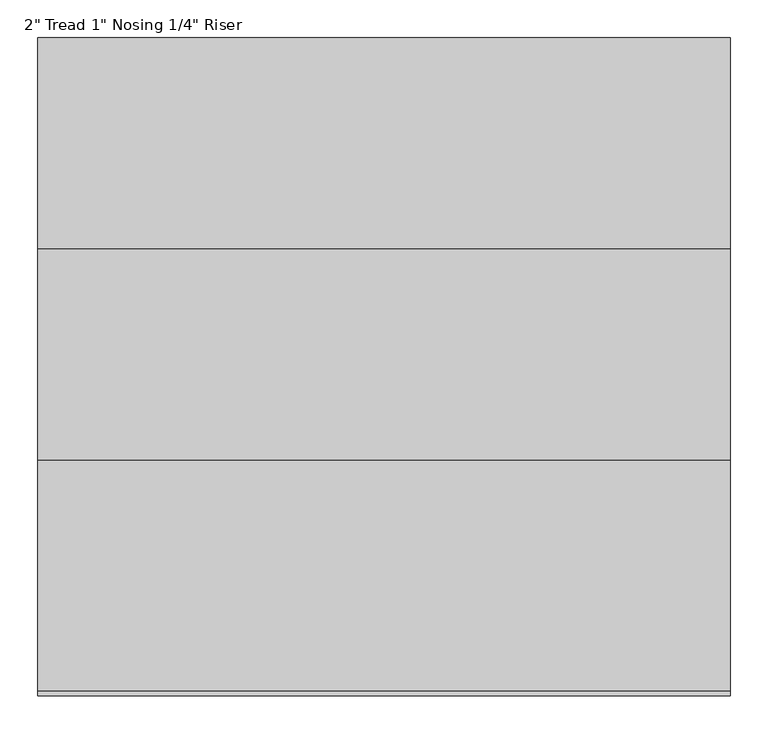
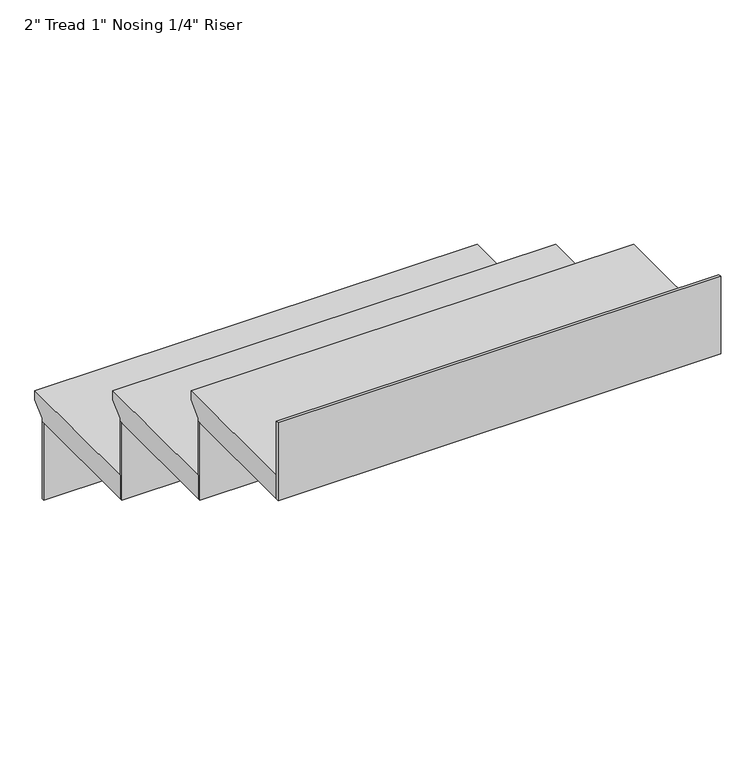
"""IFC4 building model written with IfcOpenShell, lengths in millimetres: stair flight geometry."""

from ifc_helpers import new_model, si_unit, frame, origin, place, context, project, spatial, polyline, outline, extrude, source, transform, mapped, element, save


def stair_flight_592be736(model_context):
    return source(origin(), model_context, "Body", "SweptSolid", [
        extrude(outline(polyline([(-19826.9851539, 43014.6172466), (-19522.1851539, 43014.6172466), (-19522.1851539, 42995.5672466), (-19547.5851539, 42970.1672466), (-19547.5851539, 42963.8172466), (-19826.9851539, 42963.8172466), (-19826.9851539, 43014.6172466)])), frame((-2296.6415084, 0.0, 0.0), z_axis=(1.0, 0.0, 0.0), x_axis=(0.0, 1.0, 0.0)), (0.0, 0.0, 1.0), 914.4),
        extrude(outline(polyline([(-2296.6415084, -19553.9351539), (-2296.6415084, -19547.5851539), (-1382.2415084, -19547.5851539), (-1382.2415084, -19553.9351539), (-2296.6415084, -19553.9351539)])), frame((0.0, 0.0, 42794.4839133), z_axis=(0.0, 0.0, 1.0), x_axis=(1.0, 0.0, 0.0)), (0.0, 0.0, 1.0), 169.3333333),
        extrude(outline(polyline([(-2296.6415084, -19833.3351539), (-2296.6415084, -19826.9851539), (-1382.2415084, -19826.9851539), (-1382.2415084, -19833.3351539), (-2296.6415084, -19833.3351539)])), frame((0.0, 0.0, 42963.8172466), z_axis=(0.0, 0.0, 1.0), x_axis=(1.0, 0.0, 0.0)), (0.0, 0.0, 1.0), 169.3333333),
        extrude(outline(polyline([(-20106.3851539, 43183.9505799), (-19801.5851539, 43183.9505799), (-19801.5851539, 43164.9005799), (-19826.9851539, 43139.5005799), (-19826.9851539, 43133.1505799), (-20106.3851539, 43133.1505799), (-20106.3851539, 43183.9505799)])), frame((-2296.6415084, 0.0, 0.0), z_axis=(1.0, 0.0, 0.0), x_axis=(0.0, 1.0, 0.0)), (0.0, 0.0, 1.0), 914.4),
        extrude(outline(polyline([(-2296.6415084, -20112.7351539), (-2296.6415084, -20106.3851539), (-1382.2415084, -20106.3851539), (-1382.2415084, -20112.7351539), (-2296.6415084, -20112.7351539)])), frame((0.0, 0.0, 43133.1505799), z_axis=(0.0, 0.0, 1.0), x_axis=(1.0, 0.0, 0.0)), (0.0, 0.0, 1.0), 169.3333333),
        extrude(outline(polyline([(-2296.6415084, -20392.1351539), (-2296.6415084, -20385.7851539), (-1382.2415084, -20385.7851539), (-1382.2415084, -20392.1351539), (-2296.6415084, -20392.1351539)])), frame((0.0, 0.0, 43302.4839133), z_axis=(0.0, 0.0, 1.0), x_axis=(1.0, 0.0, 0.0)), (0.0, 0.0, 1.0), 169.3333333),
        extrude(outline(polyline([(-20385.7851539, 43353.2839133), (-20080.9851539, 43353.2839133), (-20080.9851539, 43334.2339133), (-20106.3851539, 43308.8339133), (-20106.3851539, 43302.4839133), (-20385.7851539, 43302.4839133), (-20385.7851539, 43353.2839133)])), frame((-2296.6415084, 0.0, 0.0), z_axis=(1.0, 0.0, 0.0), x_axis=(0.0, 1.0, 0.0)), (0.0, 0.0, 1.0), 914.4),
    ])


if __name__ == "__main__":
    model = new_model("IFC4")
    model_context = context("Model", 3, world=origin())
    ifc_project = project(units=[si_unit("LENGTHUNIT", "METRE", prefix="MILLI")], contexts=[model_context])
    site = spatial("IfcSite", under=ifc_project)
    building = spatial("IfcBuilding", under=site)
    placement = place(None, origin())
    stair_flight_shape = stair_flight_592be736(model_context)
    element("IfcStairFlight", 1, ObjectType="2\" Tread 1\" Nosing 1/4\" Riser", at=placement, inside=building, context=model_context, shape_type="MappedRepresentation", body=[
        mapped(stair_flight_shape, transform((0.0, 0.0, 0.0), x_axis=(1.0, 0.0, 0.0), y_axis=(0.0, 1.0, 0.0), z_axis=(0.0, 0.0, 1.0))),
    ])
    save(model, "model.ifc")
